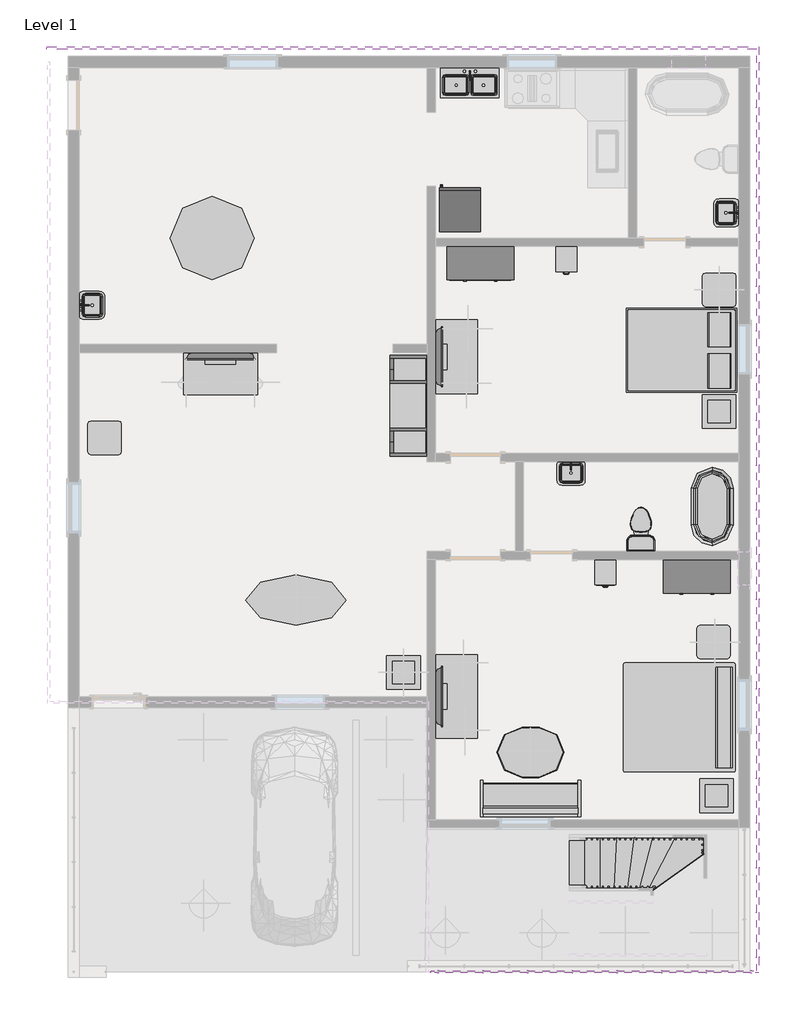
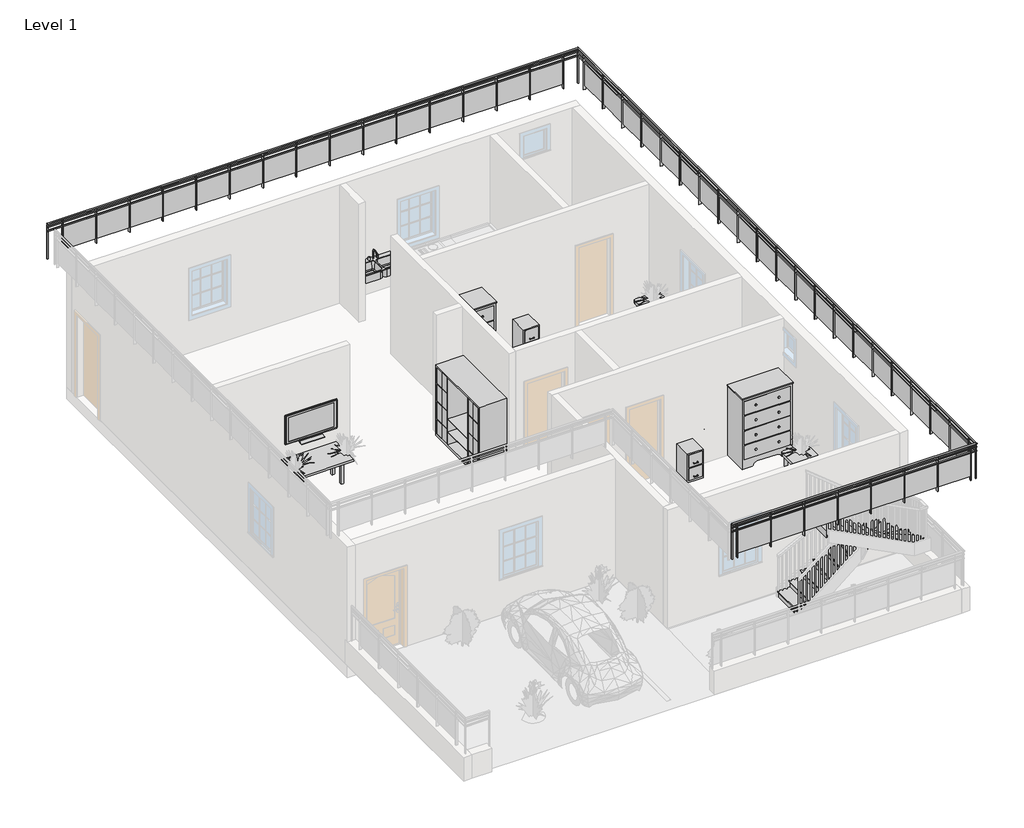
# One storey, part 4 of 5: 23 furniture elements, 7 flow terminals, 1 proxy, 1 railing, 1 stair flight.
"""IFC4 building model written with IfcOpenShell, lengths in millimetres."""

from ifc_helpers import new_model, si_unit, frame, origin, place, context, project, spatial, polyline, circle_curve, ellipse_curve, outline, extrude, faceted_brep, transform, mapped, element, save
from ifc_brep_helpers import plane_surface, cylinder_surface, advanced_brep
from components import proxy_a13a33b2, flow_terminal_accce45a, flow_terminal_a53be723, flow_terminal_62a433f7, toilet_domestic_3d_toilet_domestic_3d_f7549cf7, toilet_domestic_3d_toilet_domestic_3d_183bbd19, flow_terminal_a2f06f5b, furniture_1d2926bd, furniture_1fc5af50, furniture_bb55ed6b, furniture_9fa109b2, furniture_cf0b6580, furniture_a4ffab56, furniture_7a3aaa4f, furniture_fdf74506, furniture_b5c51a22, furniture_be1c6672, furniture_bbcc68ce, furniture_0791916c, furniture_31d08a24, furniture_48e8c7c4, furniture_2bbcfec9, stair_flight_469f198f

model = new_model("IFC4")

# Units and contexts
model_context = context("Model", 3, world=origin())
ifc_project = project(units=[si_unit("LENGTHUNIT", "METRE", prefix="MILLI")], contexts=[model_context])

# Site, building, storey
site = spatial("IfcSite", under=ifc_project)
building = spatial("IfcBuilding", under=site)
storey = spatial("IfcBuildingStorey", under=building, Name="Level 1", Elevation=0.0)

# Proxy
placement = place(None, origin())
proxy_shape = proxy_a13a33b2(model_context)
element("IfcBuildingElementProxy", 1, Name="Refrigerator : 30\" x 32\" RH", ObjectType="Refrigerator : 30\" x 32\" RH", at=placement, inside=storey, context=model_context, shape_type="MappedRepresentation", body=[
    mapped(proxy_shape, transform((-5198.8866134, 11199.3143341, 0.0), x_axis=(-1.0000000000000004, 0.0, 0.0), y_axis=(0.0, -1.0000000000000004, 0.0), z_axis=(0.0, 0.0, 1.0))),
])

# Flow terminals
flow_terminal_shape = flow_terminal_accce45a(model_context)
element("IfcFlowTerminal", 2, ObjectType="Floor Drain - Round : 5\" Strainer - 2\" Drain", at=placement, inside=storey, context=model_context, shape_type="MappedRepresentation", body=[
    mapped(flow_terminal_shape, transform((-1168.2241134, 5288.6633056, 0.0), x_axis=(1.0, 0.0, 0.0), y_axis=(0.0, 1.0, 0.0), z_axis=(0.0, 0.0, 1.0))),
])
flow_terminal_2_shape = flow_terminal_a53be723(model_context)
element("IfcFlowTerminal", 3, ObjectType="Sink Kitchen-Double : 42\" x 21\"", at=placement, inside=storey, context=model_context, shape_type="MappedRepresentation", body=[
    mapped(flow_terminal_2_shape, transform((-5032.013354, 13515.9179045, 0.0), x_axis=(1.0, 0.0, 0.0), y_axis=(0.0, 1.0, 0.0), z_axis=(0.0, 0.0, 1.0))),
])
flow_terminal_3_shape = flow_terminal_62a433f7(model_context)
element("IfcFlowTerminal", 4, ObjectType="Sink Vanity-Square : 20\" x 18\"", at=placement, inside=storey, context=model_context, shape_type="MappedRepresentation", body=[
    mapped(flow_terminal_3_shape, transform((-11935.4787123, 9463.9740651, 0.0), x_axis=(0.0, 1.0000000000000002, 0.0), y_axis=(-1.0000000000000002, 0.0, 0.0), z_axis=(0.0, 0.0, 1.0))),
])
element("IfcFlowTerminal", 5, ObjectType="Sink Vanity-Square : 20\" x 18\"", at=placement, inside=storey, context=model_context, shape_type="MappedRepresentation", body=[
    mapped(flow_terminal_3_shape, transform((-306.9695145, 11171.7525462, 0.0), x_axis=(0.0, -1.0000000000000004, 0.0), y_axis=(1.0000000000000004, 0.0, 0.0), z_axis=(0.0, 0.0, 1.0))),
])
element("IfcFlowTerminal", 6, ObjectType="Sink Vanity-Square : 20\" x 18\"", at=placement, inside=storey, context=model_context, shape_type="MappedRepresentation", body=[
    mapped(flow_terminal_3_shape, transform((-3190.513354, 6480.1179045, 0.0), x_axis=(1.0, 0.0, 0.0), y_axis=(0.0, 1.0, 0.0), z_axis=(0.0, 0.0, 1.0))),
])
toilet_domestic_3d_toilet_domestic_3d_shape = toilet_domestic_3d_toilet_domestic_3d_f7549cf7(model_context)
toilet_domestic_3d_toilet_domestic_3d_2_shape = toilet_domestic_3d_toilet_domestic_3d_183bbd19(model_context)
element("IfcFlowTerminal", 7, ObjectType="Toilet-Domestic-3D : Toilet-Domestic-3D", at=placement, inside=storey, context=model_context, shape_type="MappedRepresentation", body=[
    mapped(toilet_domestic_3d_toilet_domestic_3d_shape, transform((-1904.8241134, 5503.959333, 0.0), x_axis=(-1.0000000000000002, 0.0, 0.0), y_axis=(0.0, -1.0000000000000002, 0.0), z_axis=(0.0, 0.0, 1.0))),
    mapped(toilet_domestic_3d_toilet_domestic_3d_2_shape, transform((-1904.8241134, 5503.959333, 0.0), x_axis=(-1.0000000000000002, 0.0, 0.0), y_axis=(0.0, -1.0000000000000002, 0.0), z_axis=(0.0, 0.0, 1.0))),
])
flow_terminal_4_shape = flow_terminal_a2f06f5b(model_context)
element("IfcFlowTerminal", 8, ObjectType="Tub-Free Standing-3D : 30\" x 60\" 2", at=placement, inside=storey, context=model_context, shape_type="MappedRepresentation", body=[
    mapped(flow_terminal_4_shape, transform((-609.4241134, 5822.0633056, 0.0), x_axis=(1.0000000000000004, 0.0, 0.0), y_axis=(0.0, 1.0000000000000004, 0.0), z_axis=(0.0, 0.0, 1.0))),
])

# Furniture
furniture_shape = furniture_1d2926bd(model_context)
element("IfcFurniture", 9, ObjectType="Bed-Box : Queen 60\" x 79\"", at=placement, inside=storey, context=model_context, shape_type="MappedRepresentation", body=[
    mapped(furniture_shape, transform((-933.7946052, 8997.0633056, 0.0), x_axis=(0.0, -1.0, 0.0), y_axis=(1.0, 0.0, 0.0), z_axis=(0.0, 0.0, 1.0))),
])
furniture_2_shape = furniture_1fc5af50(model_context)
element("IfcFurniture", 10, ObjectType="Bed-Standard.0001 : King 78\" x 80\"", at=placement, inside=storey, context=model_context, shape_type="MappedRepresentation", body=[
    mapped(furniture_2_shape, transform((-1160.7290314, 2258.1518302, 0.0), x_axis=(0.0, -1.0, 0.0), y_axis=(1.0, 0.0, 0.0), z_axis=(0.0, 0.0, 1.0))),
])
furniture_3_shape = furniture_bb55ed6b(model_context)
element("IfcFurniture", 11, ObjectType="Cabinet-File 2 Drawer : 15\" x 18\"", at=placement, inside=storey, context=model_context, shape_type="MappedRepresentation", body=[
    mapped(furniture_3_shape, transform((-3135.8276664, 10459.9976058, 0.0), x_axis=(1.0, 0.0, 0.0), y_axis=(0.0, 1.0, 0.0), z_axis=(0.0, 0.0, 1.0))),
])
element("IfcFurniture", 12, ObjectType="Cabinet-File 2 Drawer : 15\" x 18\"", at=placement, inside=storey, context=model_context, shape_type="MappedRepresentation", body=[
    mapped(furniture_3_shape, transform((-2424.6276664, 4770.3976058, 0.0), x_axis=(1.0, 0.0, 0.0), y_axis=(0.0, 1.0, 0.0), z_axis=(0.0, 0.0, 1.0))),
])
furniture_4_shape = furniture_9fa109b2(model_context)
element("IfcFurniture", 13, ObjectType="Dresser : 48\" x 72\" x 24\"", at=placement, inside=storey, context=model_context, shape_type="MappedRepresentation", body=[
    mapped(furniture_4_shape, transform((-4556.6308536, 10604.8262597, 0.0), x_axis=(1.0, 0.0, 0.0), y_axis=(0.0, 1.0, 0.0), z_axis=(0.0, 0.0, 1.0))),
])
element("IfcFurniture", 14, ObjectType="Dresser : 48\" x 72\" x 24\"", at=placement, inside=storey, context=model_context, shape_type="MappedRepresentation", body=[
    mapped(furniture_4_shape, transform((-619.6308536, 4915.2262597, 0.0), x_axis=(1.0, 0.0, 0.0), y_axis=(0.0, 1.0, 0.0), z_axis=(0.0, 0.0, 1.0))),
])
furniture_5_shape = furniture_cf0b6580(model_context)
element("IfcFurniture", 15, ObjectType="Entertainment Center : 72\" x 72\" x 24\"", at=placement, inside=storey, context=model_context, shape_type="MappedRepresentation", body=[
    mapped(furniture_5_shape, transform((-5689.4241134, 7650.8633056, 0.0), x_axis=(0.0, -1.0000000000000004, 0.0), y_axis=(1.0000000000000004, 0.0, 0.0), z_axis=(0.0, 0.0, 1.0))),
])
furniture_6_shape = furniture_a4ffab56(model_context)
element("IfcFurniture", 16, ObjectType="Sofa : 72\"", at=placement, inside=storey, context=model_context, shape_type="MappedRepresentation", body=[
    mapped(furniture_6_shape, transform((-3841.0536216, 659.617404, 0.0), x_axis=(-1.0000000000000002, 0.0, 0.0), y_axis=(0.0, -1.0000000000000002, 0.0), z_axis=(0.0, 0.0, 1.0))),
])
furniture_7_shape = furniture_7a3aaa4f(model_context)
element("IfcFurniture", 17, ObjectType="TV - Flat Screen : 42\"", at=placement, inside=storey, context=model_context, shape_type="MappedRepresentation", body=[
    mapped(furniture_7_shape, transform((-5580.0854898, 8543.8078198, 990.6), x_axis=(0.0, 1.0000000000000002, 0.0), y_axis=(-1.0000000000000002, 0.0, 0.0), z_axis=(0.0, 0.0, 1.0))),
])
element("IfcFurniture", 18, ObjectType="TV - Flat Screen : 42\"", at=placement, inside=storey, context=model_context, shape_type="MappedRepresentation", body=[
    mapped(furniture_7_shape, transform((-5580.0854898, 2371.6078198, 990.6), x_axis=(0.0, 1.0000000000000002, 0.0), y_axis=(-1.0000000000000002, 0.0, 0.0), z_axis=(0.0, 0.0, 1.0))),
])
furniture_8_shape = furniture_fdf74506(model_context)
element("IfcFurniture", 19, ObjectType="TV - Flat Screen : 50\"", at=placement, inside=storey, context=model_context, shape_type="MappedRepresentation", body=[
    mapped(furniture_8_shape, transform((-9546.2795993, 8557.524682, 1041.4), x_axis=(1.0, 0.0, 0.0), y_axis=(0.0, 1.0, 0.0), z_axis=(0.0, 0.0, 1.0))),
])
furniture_9_shape = furniture_b5c51a22(model_context)
element("IfcFurniture", 20, ObjectType="Table-Coffee : 24\" x 24\" x 24\"", at=placement, inside=storey, context=model_context, shape_type="MappedRepresentation", body=[
    mapped(furniture_9_shape, transform((-500.6898801, 7454.0522278, 0.0), x_axis=(1.0, 0.0, 0.0), y_axis=(0.0, 1.0, 0.0), z_axis=(0.0, 0.0, 1.0))),
])
element("IfcFurniture", 21, ObjectType="Table-Coffee : 24\" x 24\" x 24\"", at=placement, inside=storey, context=model_context, shape_type="MappedRepresentation", body=[
    mapped(furniture_9_shape, transform((-551.4898801, 469.0522278, 0.0), x_axis=(1.0, 0.0, 0.0), y_axis=(0.0, 1.0, 0.0), z_axis=(0.0, 0.0, 1.0))),
])
element("IfcFurniture", 22, ObjectType="Table-Coffee : 24\" x 24\" x 24\"", at=placement, inside=storey, context=model_context, shape_type="MappedRepresentation", body=[
    mapped(furniture_9_shape, transform((-6241.0898801, 2710.6022278, 0.0), x_axis=(1.0, 0.0, 0.0), y_axis=(0.0, 1.0, 0.0), z_axis=(0.0, 0.0, 1.0))),
])
furniture_10_shape = furniture_be1c6672(model_context)
element("IfcFurniture", 23, ObjectType="Table-Dining Oval : 36\" x 48\"", at=placement, inside=storey, context=model_context, shape_type="MappedRepresentation", body=[
    mapped(furniture_10_shape, transform((-3509.6044413, 1709.7616663, 0.0), x_axis=(1.0, 0.0, 0.0), y_axis=(0.0, 1.0, 0.0), z_axis=(0.0, 0.0, 1.0))),
])
furniture_11_shape = furniture_bbcc68ce(model_context)
element("IfcFurniture", 24, ObjectType="Table-Dining Round w Chairs : 60\" Diameter", at=placement, inside=storey, context=model_context, shape_type="MappedRepresentation", body=[
    mapped(furniture_11_shape, transform((-9806.3060806, 10883.7419941, 0.0), x_axis=(1.0, 0.0, 0.0), y_axis=(0.0, 1.0, 0.0), z_axis=(0.0, 0.0, 1.0))),
])
furniture_12_shape = furniture_0791916c(model_context)
element("IfcFurniture", 25, ObjectType="Table-Ellipse : 72\" x 36\"", at=placement, inside=storey, context=model_context, shape_type="MappedRepresentation", body=[
    mapped(furniture_12_shape, transform((-8178.6241134, 4120.2633056, 0.0), x_axis=(1.0, 0.0, 0.0), y_axis=(0.0, 1.0, 0.0), z_axis=(0.0, 0.0, 1.0))),
])
furniture_13_shape = furniture_31d08a24(model_context)
element("IfcFurniture", 26, ObjectType="Table-End : 24\" x 24\"", at=placement, inside=storey, context=model_context, shape_type="MappedRepresentation", body=[
    mapped(furniture_13_shape, transform((-790.9577437, 9606.6633056, 0.0), x_axis=(1.0, 0.0, 0.0), y_axis=(0.0, 1.0, 0.0), z_axis=(0.0, 0.0, 1.0))),
])
element("IfcFurniture", 27, ObjectType="Table-End : 24\" x 24\"", at=placement, inside=storey, context=model_context, shape_type="MappedRepresentation", body=[
    mapped(furniture_13_shape, transform((-892.5577437, 3205.8633056, 0.0), x_axis=(1.0, 0.0, 0.0), y_axis=(0.0, 1.0, 0.0), z_axis=(0.0, 0.0, 1.0))),
])
element("IfcFurniture", 28, ObjectType="Table-End : 24\" x 24\"", at=placement, inside=storey, context=model_context, shape_type="MappedRepresentation", body=[
    mapped(furniture_13_shape, transform((-11966.9577437, 6914.2633056, 0.0), x_axis=(1.0, 0.0, 0.0), y_axis=(0.0, 1.0, 0.0), z_axis=(0.0, 0.0, 1.0))),
])
furniture_14_shape = furniture_48e8c7c4(model_context)
element("IfcFurniture", 29, ObjectType="Table-Rectangular : 72\" x 30\"", at=placement, inside=storey, context=model_context, shape_type="MappedRepresentation", body=[
    mapped(furniture_14_shape, transform((-5257.6241134, 8539.8633056, 0.0), x_axis=(0.0, 1.0000000000000002, 0.0), y_axis=(-1.0000000000000002, 0.0, 0.0), z_axis=(0.0, 0.0, 1.0))),
])
element("IfcFurniture", 30, ObjectType="Table-Rectangular : 72\" x 30\"", at=placement, inside=storey, context=model_context, shape_type="MappedRepresentation", body=[
    mapped(furniture_14_shape, transform((-9550.2241134, 8235.0633056, 0.0), x_axis=(1.0, 0.0, 0.0), y_axis=(0.0, 1.0, 0.0), z_axis=(0.0, 0.0, 1.0))),
])
furniture_15_shape = furniture_2bbcfec9(model_context)
element("IfcFurniture", 31, ObjectType="Table-Rectangular : 72\" x 30\" 2", at=placement, inside=storey, context=model_context, shape_type="MappedRepresentation", body=[
    mapped(furniture_15_shape, transform((-5257.6241134, 2367.6633056, 0.0), x_axis=(0.0, 1.0000000000000002, 0.0), y_axis=(-1.0000000000000002, 0.0, 0.0), z_axis=(0.0, 0.0, 1.0))),
])

# Railing
element("IfcRailing", 32, ObjectType="Glass Panel - Bottom Fill", at=placement, inside=storey, context=model_context, shape_type="SolidModel", body=[
    advanced_brep(
    [(-12707.5816429, 14134.2133056, 4248.15), (-12707.5816429, 14172.3133056, 4248.15), (-5722.5816429, -2617.0866944, 4248.15), (-5722.5816429, -2655.1866944, 4248.15), (201.9683571, 14134.2133056, 4248.15), (240.0683571, 14172.3133056, 4248.15), (201.9683571, -2617.0866944, 4248.15), (240.0683571, -2655.1866944, 4248.15)],
    [
        (0, 1, circle_curve(frame((-12707.5816429, 14153.2633056, 4248.15), z_axis=(-1.0, 0.0, 0.0), x_axis=(0.0, 1.0, 0.0)), 19.05)),
        (1, 0, circle_curve(frame((-12707.5816429, 14153.2633056, 4248.15), z_axis=(-1.0, 0.0, 0.0), x_axis=(0.0, 1.0, 0.0)), 19.05)),
        (2, 3, circle_curve(frame((-5722.5816429, -2636.1366944, 4248.15), z_axis=(-1.0, 0.0, 0.0), x_axis=(0.0, -1.0, 0.0)), 19.05)),
        (3, 2, circle_curve(frame((-5722.5816429, -2636.1366944, 4248.15), z_axis=(-1.0, 0.0, 0.0), x_axis=(0.0, -1.0, 0.0)), 19.05)),
        (0, 4),
        (4, 5, ellipse_curve(frame((221.0183571, 14153.2633056, 4248.15), z_axis=(-0.7071067811865459, 0.7071067811865491, 0.0), x_axis=(-0.707106781186549, -0.7071067811865458, 0.0)), 26.9407684, 19.05)),
        (5, 1),
        (5, 4, ellipse_curve(frame((221.0183571, 14153.2633056, 4248.15), z_axis=(-0.7071067811865459, 0.7071067811865491, 0.0), x_axis=(-0.707106781186549, -0.7071067811865458, 0.0)), 26.9407684, 19.05)),
        (4, 6),
        (6, 7, ellipse_curve(frame((221.0183571, -2636.1366944, 4248.15), z_axis=(0.7071067811865492, 0.7071067811865458, 0.0), x_axis=(-0.7071067811865457, 0.7071067811865495, 0.0)), 26.9407684, 19.05)),
        (7, 5),
        (7, 6, ellipse_curve(frame((221.0183571, -2636.1366944, 4248.15), z_axis=(0.7071067811865492, 0.7071067811865458, 0.0), x_axis=(-0.7071067811865457, 0.7071067811865495, 0.0)), 26.9407684, 19.05)),
        (6, 2),
        (3, 7),
    ],
    [
        plane_surface(frame((-12707.5816429, 14153.2633056, 4267.2), z_axis=(-1.0, 0.0, 0.0), x_axis=(0.0, 1.0, 0.0))),
        plane_surface(frame((-5722.5816429, -2636.1366944, 4267.2), z_axis=(-1.0, 0.0, 0.0), x_axis=(0.0, -1.0, 0.0))),
        cylinder_surface(frame((-12707.5816429, 14153.2633056, 4248.15), z_axis=(-1.0, 0.0, 0.0), x_axis=(0.0, 1.0, 0.0)), 19.05),
        cylinder_surface(frame((221.0183571, 14153.2633056, 4248.15), z_axis=(0.0, 1.0, 0.0), x_axis=(1.0, 0.0, 0.0)), 19.05),
        cylinder_surface(frame((221.0183571, -2636.1366944, 4248.15), z_axis=(1.0, 0.0, 0.0), x_axis=(0.0, -1.0, 0.0)), 19.05),
    ],
    [
        (0, [[1, 2]]),
        (1, [[3, 4]]),
        (2, [[-1, 5, 6, 7]]),
        (2, [[-2, -7, 8, -5]]),
        (3, [[-6, 9, 10, 11]]),
        (3, [[-8, -11, 12, -9]]),
        (4, [[-10, 13, -4, 14]]),
        (4, [[-12, -14, -3, -13]]),
    ],
),
    faceted_brep([(-12707.5816429, 14140.5633056, 4178.3), (-12707.5816429, 14165.9633056, 4178.3), (-12707.5816429, 14165.9633056, 4152.9), (-12707.5816429, 14140.5633056, 4152.9), (208.3183571, 14140.5633056, 4178.3), (233.7183571, 14165.9633056, 4178.3), (233.7183571, 14165.9633056, 4152.9), (208.3183571, 14140.5633056, 4152.9), (208.3183571, -2623.4366944, 4178.3), (233.7183571, -2648.8366944, 4178.3), (233.7183571, -2648.8366944, 4152.9), (208.3183571, -2623.4366944, 4152.9), (-5722.5816429, -2623.4366944, 4178.3), (-5722.5816429, -2623.4366944, 4152.9), (-5722.5816429, -2648.8366944, 4152.9), (-5722.5816429, -2648.8366944, 4178.3)], [[[0, 1, 2, 3]], [[1, 0, 4, 5]], [[2, 1, 5, 6]], [[3, 2, 6, 7]], [[0, 3, 7, 4]], [[5, 4, 8, 9]], [[6, 5, 9, 10]], [[7, 6, 10, 11]], [[4, 7, 11, 8]], [[12, 13, 14, 15]], [[9, 8, 12, 15]], [[10, 9, 15, 14]], [[11, 10, 14, 13]], [[8, 11, 13, 12]]]),
    faceted_brep([(-12707.5816429, 14140.5633056, 4076.7), (-12707.5816429, 14165.9633056, 4076.7), (-12707.5816429, 14165.9633056, 4051.3), (-12707.5816429, 14140.5633056, 4051.3), (208.3183571, 14140.5633056, 4076.7), (233.7183571, 14165.9633056, 4076.7), (233.7183571, 14165.9633056, 4051.3), (208.3183571, 14140.5633056, 4051.3), (208.3183571, -2623.4366944, 4076.7), (233.7183571, -2648.8366944, 4076.7), (233.7183571, -2648.8366944, 4051.3), (208.3183571, -2623.4366944, 4051.3), (-5722.5816429, -2623.4366944, 4076.7), (-5722.5816429, -2623.4366944, 4051.3), (-5722.5816429, -2648.8366944, 4051.3), (-5722.5816429, -2648.8366944, 4076.7)], [[[0, 1, 2, 3]], [[1, 0, 4, 5]], [[2, 1, 5, 6]], [[3, 2, 6, 7]], [[0, 3, 7, 4]], [[5, 4, 8, 9]], [[6, 5, 9, 10]], [[7, 6, 10, 11]], [[4, 7, 11, 8]], [[12, 13, 14, 15]], [[9, 8, 12, 15]], [[10, 9, 15, 14]], [[11, 10, 14, 13]], [[8, 11, 13, 12]]]),
    extrude(outline(polyline([(-5589.2316429, -2610.7366944), (-5589.2316429, -2661.5366944), (-5601.9316429, -2661.5366944), (-5601.9316429, -2610.7366944), (-5589.2316429, -2610.7366944)])), frame((0.0, 0.0, 3352.8), z_axis=(0.0, 0.0, 1.0), x_axis=(1.0, 0.0, 0.0)), (0.0, 0.0, 1.0), 876.3),
    extrude(outline(polyline([(-4782.7816429, -2642.6718514), (-5595.5816429, -2642.6718514), (-5595.5816429, -2636.3218514), (-4782.7816429, -2636.3218514), (-4782.7816429, -2642.6718514)])), frame((0.0, 0.0, 3454.4), z_axis=(0.0, 0.0, 1.0), x_axis=(1.0, 0.0, 0.0)), (0.0, 0.0, 1.0), 596.9),
    extrude(outline(polyline([(-4776.4316429, -2610.7366944), (-4776.4316429, -2661.5366944), (-4789.1316429, -2661.5366944), (-4789.1316429, -2610.7366944), (-4776.4316429, -2610.7366944)])), frame((0.0, 0.0, 3352.8), z_axis=(0.0, 0.0, 1.0), x_axis=(1.0, 0.0, 0.0)), (0.0, 0.0, 1.0), 876.3),
    extrude(outline(polyline([(-3969.9816429, -2642.6718514), (-4782.7816429, -2642.6718514), (-4782.7816429, -2636.3218514), (-3969.9816429, -2636.3218514), (-3969.9816429, -2642.6718514)])), frame((0.0, 0.0, 3454.4), z_axis=(0.0, 0.0, 1.0), x_axis=(1.0, 0.0, 0.0)), (0.0, 0.0, 1.0), 596.9),
    extrude(outline(polyline([(-3963.6316429, -2610.7366944), (-3963.6316429, -2661.5366944), (-3976.3316429, -2661.5366944), (-3976.3316429, -2610.7366944), (-3963.6316429, -2610.7366944)])), frame((0.0, 0.0, 3352.8), z_axis=(0.0, 0.0, 1.0), x_axis=(1.0, 0.0, 0.0)), (0.0, 0.0, 1.0), 876.3),
    extrude(outline(polyline([(-3157.1816429, -2642.6718514), (-3969.9816429, -2642.6718514), (-3969.9816429, -2636.3218514), (-3157.1816429, -2636.3218514), (-3157.1816429, -2642.6718514)])), frame((0.0, 0.0, 3454.4), z_axis=(0.0, 0.0, 1.0), x_axis=(1.0, 0.0, 0.0)), (0.0, 0.0, 1.0), 596.9),
    extrude(outline(polyline([(-3150.8316429, -2610.7366944), (-3150.8316429, -2661.5366944), (-3163.5316429, -2661.5366944), (-3163.5316429, -2610.7366944), (-3150.8316429, -2610.7366944)])), frame((0.0, 0.0, 3352.8), z_axis=(0.0, 0.0, 1.0), x_axis=(1.0, 0.0, 0.0)), (0.0, 0.0, 1.0), 876.3),
    extrude(outline(polyline([(-2344.3816429, -2642.6718514), (-3157.1816429, -2642.6718514), (-3157.1816429, -2636.3218514), (-2344.3816429, -2636.3218514), (-2344.3816429, -2642.6718514)])), frame((0.0, 0.0, 3454.4), z_axis=(0.0, 0.0, 1.0), x_axis=(1.0, 0.0, 0.0)), (0.0, 0.0, 1.0), 596.9),
    extrude(outline(polyline([(-2338.0316429, -2610.7366944), (-2338.0316429, -2661.5366944), (-2350.7316429, -2661.5366944), (-2350.7316429, -2610.7366944), (-2338.0316429, -2610.7366944)])), frame((0.0, 0.0, 3352.8), z_axis=(0.0, 0.0, 1.0), x_axis=(1.0, 0.0, 0.0)), (0.0, 0.0, 1.0), 876.3),
    extrude(outline(polyline([(-1531.5816429, -2642.6718514), (-2344.3816429, -2642.6718514), (-2344.3816429, -2636.3218514), (-1531.5816429, -2636.3218514), (-1531.5816429, -2642.6718514)])), frame((0.0, 0.0, 3454.4), z_axis=(0.0, 0.0, 1.0), x_axis=(1.0, 0.0, 0.0)), (0.0, 0.0, 1.0), 596.9),
    extrude(outline(polyline([(-1525.2316429, -2610.7366944), (-1525.2316429, -2661.5366944), (-1537.9316429, -2661.5366944), (-1537.9316429, -2610.7366944), (-1525.2316429, -2610.7366944)])), frame((0.0, 0.0, 3352.8), z_axis=(0.0, 0.0, 1.0), x_axis=(1.0, 0.0, 0.0)), (0.0, 0.0, 1.0), 876.3),
    extrude(outline(polyline([(-718.7816429, -2642.6718514), (-1531.5816429, -2642.6718514), (-1531.5816429, -2636.3218514), (-718.7816429, -2636.3218514), (-718.7816429, -2642.6718514)])), frame((0.0, 0.0, 3454.4), z_axis=(0.0, 0.0, 1.0), x_axis=(1.0, 0.0, 0.0)), (0.0, 0.0, 1.0), 596.9),
    extrude(outline(polyline([(-712.4316429, -2610.7366944), (-712.4316429, -2661.5366944), (-725.1316429, -2661.5366944), (-725.1316429, -2610.7366944), (-712.4316429, -2610.7366944)])), frame((0.0, 0.0, 3352.8), z_axis=(0.0, 0.0, 1.0), x_axis=(1.0, 0.0, 0.0)), (0.0, 0.0, 1.0), 876.3),
    extrude(outline(polyline([(94.0183571, -2642.6718514), (-718.7816429, -2642.6718514), (-718.7816429, -2636.3218514), (94.0183571, -2636.3218514), (94.0183571, -2642.6718514)])), frame((0.0, 0.0, 3454.4), z_axis=(0.0, 0.0, 1.0), x_axis=(1.0, 0.0, 0.0)), (0.0, 0.0, 1.0), 596.9),
    extrude(outline(polyline([(100.3683571, -2610.7366944), (100.3683571, -2661.5366944), (87.6683571, -2661.5366944), (87.6683571, -2610.7366944), (100.3683571, -2610.7366944)])), frame((0.0, 0.0, 3352.8), z_axis=(0.0, 0.0, 1.0), x_axis=(1.0, 0.0, 0.0)), (0.0, 0.0, 1.0), 876.3),
    extrude(outline(polyline([(195.6183571, -2363.0866944), (246.4183571, -2363.0866944), (246.4183571, -2375.7866944), (195.6183571, -2375.7866944), (195.6183571, -2363.0866944)])), frame((0.0, 0.0, 3352.8), z_axis=(0.0, 0.0, 1.0), x_axis=(1.0, 0.0, 0.0)), (0.0, 0.0, 1.0), 876.3),
    extrude(outline(polyline([(227.5535141, -1556.6366944), (227.5535141, -2369.4366944), (221.2035141, -2369.4366944), (221.2035141, -1556.6366944), (227.5535141, -1556.6366944)])), frame((0.0, 0.0, 3454.4), z_axis=(0.0, 0.0, 1.0), x_axis=(1.0, 0.0, 0.0)), (0.0, 0.0, 1.0), 596.9),
    extrude(outline(polyline([(195.6183571, -1550.2866944), (246.4183571, -1550.2866944), (246.4183571, -1562.9866944), (195.6183571, -1562.9866944), (195.6183571, -1550.2866944)])), frame((0.0, 0.0, 3352.8), z_axis=(0.0, 0.0, 1.0), x_axis=(1.0, 0.0, 0.0)), (0.0, 0.0, 1.0), 876.3),
    extrude(outline(polyline([(227.5535141, -743.8366944), (227.5535141, -1556.6366944), (221.2035141, -1556.6366944), (221.2035141, -743.8366944), (227.5535141, -743.8366944)])), frame((0.0, 0.0, 3454.4), z_axis=(0.0, 0.0, 1.0), x_axis=(1.0, 0.0, 0.0)), (0.0, 0.0, 1.0), 596.9),
    extrude(outline(polyline([(195.6183571, -737.4866944), (246.4183571, -737.4866944), (246.4183571, -750.1866944), (195.6183571, -750.1866944), (195.6183571, -737.4866944)])), frame((0.0, 0.0, 3352.8), z_axis=(0.0, 0.0, 1.0), x_axis=(1.0, 0.0, 0.0)), (0.0, 0.0, 1.0), 876.3),
    extrude(outline(polyline([(227.5535141, 68.9633056), (227.5535141, -743.8366944), (221.2035141, -743.8366944), (221.2035141, 68.9633056), (227.5535141, 68.9633056)])), frame((0.0, 0.0, 3454.4), z_axis=(0.0, 0.0, 1.0), x_axis=(1.0, 0.0, 0.0)), (0.0, 0.0, 1.0), 596.9),
    extrude(outline(polyline([(195.6183571, 75.3133056), (246.4183571, 75.3133056), (246.4183571, 62.6133056), (195.6183571, 62.6133056), (195.6183571, 75.3133056)])), frame((0.0, 0.0, 3352.8), z_axis=(0.0, 0.0, 1.0), x_axis=(1.0, 0.0, 0.0)), (0.0, 0.0, 1.0), 876.3),
    extrude(outline(polyline([(227.5535141, 881.7633056), (227.5535141, 68.9633056), (221.2035141, 68.9633056), (221.2035141, 881.7633056), (227.5535141, 881.7633056)])), frame((0.0, 0.0, 3454.4), z_axis=(0.0, 0.0, 1.0), x_axis=(1.0, 0.0, 0.0)), (0.0, 0.0, 1.0), 596.9),
    extrude(outline(polyline([(195.6183571, 888.1133056), (246.4183571, 888.1133056), (246.4183571, 875.4133056), (195.6183571, 875.4133056), (195.6183571, 888.1133056)])), frame((0.0, 0.0, 3352.8), z_axis=(0.0, 0.0, 1.0), x_axis=(1.0, 0.0, 0.0)), (0.0, 0.0, 1.0), 876.3),
    extrude(outline(polyline([(227.5535141, 1694.5633056), (227.5535141, 881.7633056), (221.2035141, 881.7633056), (221.2035141, 1694.5633056), (227.5535141, 1694.5633056)])), frame((0.0, 0.0, 3454.4), z_axis=(0.0, 0.0, 1.0), x_axis=(1.0, 0.0, 0.0)), (0.0, 0.0, 1.0), 596.9),
    extrude(outline(polyline([(195.6183571, 1700.9133056), (246.4183571, 1700.9133056), (246.4183571, 1688.2133056), (195.6183571, 1688.2133056), (195.6183571, 1700.9133056)])), frame((0.0, 0.0, 3352.8), z_axis=(0.0, 0.0, 1.0), x_axis=(1.0, 0.0, 0.0)), (0.0, 0.0, 1.0), 876.3),
    extrude(outline(polyline([(227.5535141, 2507.3633056), (227.5535141, 1694.5633056), (221.2035141, 1694.5633056), (221.2035141, 2507.3633056), (227.5535141, 2507.3633056)])), frame((0.0, 0.0, 3454.4), z_axis=(0.0, 0.0, 1.0), x_axis=(1.0, 0.0, 0.0)), (0.0, 0.0, 1.0), 596.9),
    extrude(outline(polyline([(195.6183571, 2513.7133056), (246.4183571, 2513.7133056), (246.4183571, 2501.0133056), (195.6183571, 2501.0133056), (195.6183571, 2513.7133056)])), frame((0.0, 0.0, 3352.8), z_axis=(0.0, 0.0, 1.0), x_axis=(1.0, 0.0, 0.0)), (0.0, 0.0, 1.0), 876.3),
    extrude(outline(polyline([(227.5535141, 3320.1633056), (227.5535141, 2507.3633056), (221.2035141, 2507.3633056), (221.2035141, 3320.1633056), (227.5535141, 3320.1633056)])), frame((0.0, 0.0, 3454.4), z_axis=(0.0, 0.0, 1.0), x_axis=(1.0, 0.0, 0.0)), (0.0, 0.0, 1.0), 596.9),
    extrude(outline(polyline([(195.6183571, 3326.5133056), (246.4183571, 3326.5133056), (246.4183571, 3313.8133056), (195.6183571, 3313.8133056), (195.6183571, 3326.5133056)])), frame((0.0, 0.0, 3352.8), z_axis=(0.0, 0.0, 1.0), x_axis=(1.0, 0.0, 0.0)), (0.0, 0.0, 1.0), 876.3),
    extrude(outline(polyline([(227.5535141, 4132.9633056), (227.5535141, 3320.1633056), (221.2035141, 3320.1633056), (221.2035141, 4132.9633056), (227.5535141, 4132.9633056)])), frame((0.0, 0.0, 3454.4), z_axis=(0.0, 0.0, 1.0), x_axis=(1.0, 0.0, 0.0)), (0.0, 0.0, 1.0), 596.9),
    extrude(outline(polyline([(195.6183571, 4139.3133056), (246.4183571, 4139.3133056), (246.4183571, 4126.6133056), (195.6183571, 4126.6133056), (195.6183571, 4139.3133056)])), frame((0.0, 0.0, 3352.8), z_axis=(0.0, 0.0, 1.0), x_axis=(1.0, 0.0, 0.0)), (0.0, 0.0, 1.0), 876.3),
    extrude(outline(polyline([(227.5535141, 4945.7633056), (227.5535141, 4132.9633056), (221.2035141, 4132.9633056), (221.2035141, 4945.7633056), (227.5535141, 4945.7633056)])), frame((0.0, 0.0, 3454.4), z_axis=(0.0, 0.0, 1.0), x_axis=(1.0, 0.0, 0.0)), (0.0, 0.0, 1.0), 596.9),
    extrude(outline(polyline([(195.6183571, 4952.1133056), (246.4183571, 4952.1133056), (246.4183571, 4939.4133056), (195.6183571, 4939.4133056), (195.6183571, 4952.1133056)])), frame((0.0, 0.0, 3352.8), z_axis=(0.0, 0.0, 1.0), x_axis=(1.0, 0.0, 0.0)), (0.0, 0.0, 1.0), 876.3),
    extrude(outline(polyline([(227.5535141, 5758.5633056), (227.5535141, 4945.7633056), (221.2035141, 4945.7633056), (221.2035141, 5758.5633056), (227.5535141, 5758.5633056)])), frame((0.0, 0.0, 3454.4), z_axis=(0.0, 0.0, 1.0), x_axis=(1.0, 0.0, 0.0)), (0.0, 0.0, 1.0), 596.9),
    extrude(outline(polyline([(195.6183571, 5764.9133056), (246.4183571, 5764.9133056), (246.4183571, 5752.2133056), (195.6183571, 5752.2133056), (195.6183571, 5764.9133056)])), frame((0.0, 0.0, 3352.8), z_axis=(0.0, 0.0, 1.0), x_axis=(1.0, 0.0, 0.0)), (0.0, 0.0, 1.0), 876.3),
    extrude(outline(polyline([(227.5535141, 6571.3633056), (227.5535141, 5758.5633056), (221.2035141, 5758.5633056), (221.2035141, 6571.3633056), (227.5535141, 6571.3633056)])), frame((0.0, 0.0, 3454.4), z_axis=(0.0, 0.0, 1.0), x_axis=(1.0, 0.0, 0.0)), (0.0, 0.0, 1.0), 596.9),
    extrude(outline(polyline([(195.6183571, 6577.7133056), (246.4183571, 6577.7133056), (246.4183571, 6565.0133056), (195.6183571, 6565.0133056), (195.6183571, 6577.7133056)])), frame((0.0, 0.0, 3352.8), z_axis=(0.0, 0.0, 1.0), x_axis=(1.0, 0.0, 0.0)), (0.0, 0.0, 1.0), 876.3),
    extrude(outline(polyline([(227.5535141, 7384.1633056), (227.5535141, 6571.3633056), (221.2035141, 6571.3633056), (221.2035141, 7384.1633056), (227.5535141, 7384.1633056)])), frame((0.0, 0.0, 3454.4), z_axis=(0.0, 0.0, 1.0), x_axis=(1.0, 0.0, 0.0)), (0.0, 0.0, 1.0), 596.9),
    extrude(outline(polyline([(195.6183571, 7390.5133056), (246.4183571, 7390.5133056), (246.4183571, 7377.8133056), (195.6183571, 7377.8133056), (195.6183571, 7390.5133056)])), frame((0.0, 0.0, 3352.8), z_axis=(0.0, 0.0, 1.0), x_axis=(1.0, 0.0, 0.0)), (0.0, 0.0, 1.0), 876.3),
    extrude(outline(polyline([(227.5535141, 8196.9633056), (227.5535141, 7384.1633056), (221.2035141, 7384.1633056), (221.2035141, 8196.9633056), (227.5535141, 8196.9633056)])), frame((0.0, 0.0, 3454.4), z_axis=(0.0, 0.0, 1.0), x_axis=(1.0, 0.0, 0.0)), (0.0, 0.0, 1.0), 596.9),
    extrude(outline(polyline([(195.6183571, 8203.3133056), (246.4183571, 8203.3133056), (246.4183571, 8190.6133056), (195.6183571, 8190.6133056), (195.6183571, 8203.3133056)])), frame((0.0, 0.0, 3352.8), z_axis=(0.0, 0.0, 1.0), x_axis=(1.0, 0.0, 0.0)), (0.0, 0.0, 1.0), 876.3),
    extrude(outline(polyline([(227.5535141, 9009.7633056), (227.5535141, 8196.9633056), (221.2035141, 8196.9633056), (221.2035141, 9009.7633056), (227.5535141, 9009.7633056)])), frame((0.0, 0.0, 3454.4), z_axis=(0.0, 0.0, 1.0), x_axis=(1.0, 0.0, 0.0)), (0.0, 0.0, 1.0), 596.9),
    extrude(outline(polyline([(195.6183571, 9016.1133056), (246.4183571, 9016.1133056), (246.4183571, 9003.4133056), (195.6183571, 9003.4133056), (195.6183571, 9016.1133056)])), frame((0.0, 0.0, 3352.8), z_axis=(0.0, 0.0, 1.0), x_axis=(1.0, 0.0, 0.0)), (0.0, 0.0, 1.0), 876.3),
    extrude(outline(polyline([(227.5535141, 9822.5633056), (227.5535141, 9009.7633056), (221.2035141, 9009.7633056), (221.2035141, 9822.5633056), (227.5535141, 9822.5633056)])), frame((0.0, 0.0, 3454.4), z_axis=(0.0, 0.0, 1.0), x_axis=(1.0, 0.0, 0.0)), (0.0, 0.0, 1.0), 596.9),
    extrude(outline(polyline([(195.6183571, 9828.9133056), (246.4183571, 9828.9133056), (246.4183571, 9816.2133056), (195.6183571, 9816.2133056), (195.6183571, 9828.9133056)])), frame((0.0, 0.0, 3352.8), z_axis=(0.0, 0.0, 1.0), x_axis=(1.0, 0.0, 0.0)), (0.0, 0.0, 1.0), 876.3),
    extrude(outline(polyline([(227.5535141, 10635.3633056), (227.5535141, 9822.5633056), (221.2035141, 9822.5633056), (221.2035141, 10635.3633056), (227.5535141, 10635.3633056)])), frame((0.0, 0.0, 3454.4), z_axis=(0.0, 0.0, 1.0), x_axis=(1.0, 0.0, 0.0)), (0.0, 0.0, 1.0), 596.9),
    extrude(outline(polyline([(195.6183571, 10641.7133056), (246.4183571, 10641.7133056), (246.4183571, 10629.0133056), (195.6183571, 10629.0133056), (195.6183571, 10641.7133056)])), frame((0.0, 0.0, 3352.8), z_axis=(0.0, 0.0, 1.0), x_axis=(1.0, 0.0, 0.0)), (0.0, 0.0, 1.0), 876.3),
    extrude(outline(polyline([(227.5535141, 11448.1633056), (227.5535141, 10635.3633056), (221.2035141, 10635.3633056), (221.2035141, 11448.1633056), (227.5535141, 11448.1633056)])), frame((0.0, 0.0, 3454.4), z_axis=(0.0, 0.0, 1.0), x_axis=(1.0, 0.0, 0.0)), (0.0, 0.0, 1.0), 596.9),
    extrude(outline(polyline([(195.6183571, 11454.5133056), (246.4183571, 11454.5133056), (246.4183571, 11441.8133056), (195.6183571, 11441.8133056), (195.6183571, 11454.5133056)])), frame((0.0, 0.0, 3352.8), z_axis=(0.0, 0.0, 1.0), x_axis=(1.0, 0.0, 0.0)), (0.0, 0.0, 1.0), 876.3),
    extrude(outline(polyline([(227.5535141, 12260.9633056), (227.5535141, 11448.1633056), (221.2035141, 11448.1633056), (221.2035141, 12260.9633056), (227.5535141, 12260.9633056)])), frame((0.0, 0.0, 3454.4), z_axis=(0.0, 0.0, 1.0), x_axis=(1.0, 0.0, 0.0)), (0.0, 0.0, 1.0), 596.9),
    extrude(outline(polyline([(195.6183571, 12267.3133056), (246.4183571, 12267.3133056), (246.4183571, 12254.6133056), (195.6183571, 12254.6133056), (195.6183571, 12267.3133056)])), frame((0.0, 0.0, 3352.8), z_axis=(0.0, 0.0, 1.0), x_axis=(1.0, 0.0, 0.0)), (0.0, 0.0, 1.0), 876.3),
    extrude(outline(polyline([(227.5535141, 13073.7633056), (227.5535141, 12260.9633056), (221.2035141, 12260.9633056), (221.2035141, 13073.7633056), (227.5535141, 13073.7633056)])), frame((0.0, 0.0, 3454.4), z_axis=(0.0, 0.0, 1.0), x_axis=(1.0, 0.0, 0.0)), (0.0, 0.0, 1.0), 596.9),
    extrude(outline(polyline([(195.6183571, 13080.1133056), (246.4183571, 13080.1133056), (246.4183571, 13067.4133056), (195.6183571, 13067.4133056), (195.6183571, 13080.1133056)])), frame((0.0, 0.0, 3352.8), z_axis=(0.0, 0.0, 1.0), x_axis=(1.0, 0.0, 0.0)), (0.0, 0.0, 1.0), 876.3),
    extrude(outline(polyline([(227.5535141, 13886.5633056), (227.5535141, 13073.7633056), (221.2035141, 13073.7633056), (221.2035141, 13886.5633056), (227.5535141, 13886.5633056)])), frame((0.0, 0.0, 3454.4), z_axis=(0.0, 0.0, 1.0), x_axis=(1.0, 0.0, 0.0)), (0.0, 0.0, 1.0), 596.9),
    extrude(outline(polyline([(195.6183571, 13892.9133056), (246.4183571, 13892.9133056), (246.4183571, 13880.2133056), (195.6183571, 13880.2133056), (195.6183571, 13892.9133056)])), frame((0.0, 0.0, 3352.8), z_axis=(0.0, 0.0, 1.0), x_axis=(1.0, 0.0, 0.0)), (0.0, 0.0, 1.0), 876.3),
    extrude(outline(polyline([(-153.6316429, 14127.8633056), (-153.6316429, 14178.6633056), (-140.9316429, 14178.6633056), (-140.9316429, 14127.8633056), (-153.6316429, 14127.8633056)])), frame((0.0, 0.0, 3352.8), z_axis=(0.0, 0.0, 1.0), x_axis=(1.0, 0.0, 0.0)), (0.0, 0.0, 1.0), 876.3),
    extrude(outline(polyline([(-960.0816429, 14159.7984626), (-147.2816429, 14159.7984626), (-147.2816429, 14153.4484626), (-960.0816429, 14153.4484626), (-960.0816429, 14159.7984626)])), frame((0.0, 0.0, 3454.4), z_axis=(0.0, 0.0, 1.0), x_axis=(1.0, 0.0, 0.0)), (0.0, 0.0, 1.0), 596.9),
    extrude(outline(polyline([(-966.4316429, 14127.8633056), (-966.4316429, 14178.6633056), (-953.7316429, 14178.6633056), (-953.7316429, 14127.8633056), (-966.4316429, 14127.8633056)])), frame((0.0, 0.0, 3352.8), z_axis=(0.0, 0.0, 1.0), x_axis=(1.0, 0.0, 0.0)), (0.0, 0.0, 1.0), 876.3),
    extrude(outline(polyline([(-1772.8816429, 14159.7984626), (-960.0816429, 14159.7984626), (-960.0816429, 14153.4484626), (-1772.8816429, 14153.4484626), (-1772.8816429, 14159.7984626)])), frame((0.0, 0.0, 3454.4), z_axis=(0.0, 0.0, 1.0), x_axis=(1.0, 0.0, 0.0)), (0.0, 0.0, 1.0), 596.9),
    extrude(outline(polyline([(-1779.2316429, 14127.8633056), (-1779.2316429, 14178.6633056), (-1766.5316429, 14178.6633056), (-1766.5316429, 14127.8633056), (-1779.2316429, 14127.8633056)])), frame((0.0, 0.0, 3352.8), z_axis=(0.0, 0.0, 1.0), x_axis=(1.0, 0.0, 0.0)), (0.0, 0.0, 1.0), 876.3),
    extrude(outline(polyline([(-2585.6816429, 14159.7984626), (-1772.8816429, 14159.7984626), (-1772.8816429, 14153.4484626), (-2585.6816429, 14153.4484626), (-2585.6816429, 14159.7984626)])), frame((0.0, 0.0, 3454.4), z_axis=(0.0, 0.0, 1.0), x_axis=(1.0, 0.0, 0.0)), (0.0, 0.0, 1.0), 596.9),
    extrude(outline(polyline([(-2592.0316429, 14127.8633056), (-2592.0316429, 14178.6633056), (-2579.3316429, 14178.6633056), (-2579.3316429, 14127.8633056), (-2592.0316429, 14127.8633056)])), frame((0.0, 0.0, 3352.8), z_axis=(0.0, 0.0, 1.0), x_axis=(1.0, 0.0, 0.0)), (0.0, 0.0, 1.0), 876.3),
    extrude(outline(polyline([(-3398.4816429, 14159.7984626), (-2585.6816429, 14159.7984626), (-2585.6816429, 14153.4484626), (-3398.4816429, 14153.4484626), (-3398.4816429, 14159.7984626)])), frame((0.0, 0.0, 3454.4), z_axis=(0.0, 0.0, 1.0), x_axis=(1.0, 0.0, 0.0)), (0.0, 0.0, 1.0), 596.9),
    extrude(outline(polyline([(-3404.8316429, 14127.8633056), (-3404.8316429, 14178.6633056), (-3392.1316429, 14178.6633056), (-3392.1316429, 14127.8633056), (-3404.8316429, 14127.8633056)])), frame((0.0, 0.0, 3352.8), z_axis=(0.0, 0.0, 1.0), x_axis=(1.0, 0.0, 0.0)), (0.0, 0.0, 1.0), 876.3),
    extrude(outline(polyline([(-4211.2816429, 14159.7984626), (-3398.4816429, 14159.7984626), (-3398.4816429, 14153.4484626), (-4211.2816429, 14153.4484626), (-4211.2816429, 14159.7984626)])), frame((0.0, 0.0, 3454.4), z_axis=(0.0, 0.0, 1.0), x_axis=(1.0, 0.0, 0.0)), (0.0, 0.0, 1.0), 596.9),
    extrude(outline(polyline([(-4217.6316429, 14127.8633056), (-4217.6316429, 14178.6633056), (-4204.9316429, 14178.6633056), (-4204.9316429, 14127.8633056), (-4217.6316429, 14127.8633056)])), frame((0.0, 0.0, 3352.8), z_axis=(0.0, 0.0, 1.0), x_axis=(1.0, 0.0, 0.0)), (0.0, 0.0, 1.0), 876.3),
    extrude(outline(polyline([(-5024.0816429, 14159.7984626), (-4211.2816429, 14159.7984626), (-4211.2816429, 14153.4484626), (-5024.0816429, 14153.4484626), (-5024.0816429, 14159.7984626)])), frame((0.0, 0.0, 3454.4), z_axis=(0.0, 0.0, 1.0), x_axis=(1.0, 0.0, 0.0)), (0.0, 0.0, 1.0), 596.9),
    extrude(outline(polyline([(-5030.4316429, 14127.8633056), (-5030.4316429, 14178.6633056), (-5017.7316429, 14178.6633056), (-5017.7316429, 14127.8633056), (-5030.4316429, 14127.8633056)])), frame((0.0, 0.0, 3352.8), z_axis=(0.0, 0.0, 1.0), x_axis=(1.0, 0.0, 0.0)), (0.0, 0.0, 1.0), 876.3),
    extrude(outline(polyline([(-5836.8816429, 14159.7984626), (-5024.0816429, 14159.7984626), (-5024.0816429, 14153.4484626), (-5836.8816429, 14153.4484626), (-5836.8816429, 14159.7984626)])), frame((0.0, 0.0, 3454.4), z_axis=(0.0, 0.0, 1.0), x_axis=(1.0, 0.0, 0.0)), (0.0, 0.0, 1.0), 596.9),
    extrude(outline(polyline([(-5843.2316429, 14127.8633056), (-5843.2316429, 14178.6633056), (-5830.5316429, 14178.6633056), (-5830.5316429, 14127.8633056), (-5843.2316429, 14127.8633056)])), frame((0.0, 0.0, 3352.8), z_axis=(0.0, 0.0, 1.0), x_axis=(1.0, 0.0, 0.0)), (0.0, 0.0, 1.0), 876.3),
    extrude(outline(polyline([(-6649.6816429, 14159.7984626), (-5836.8816429, 14159.7984626), (-5836.8816429, 14153.4484626), (-6649.6816429, 14153.4484626), (-6649.6816429, 14159.7984626)])), frame((0.0, 0.0, 3454.4), z_axis=(0.0, 0.0, 1.0), x_axis=(1.0, 0.0, 0.0)), (0.0, 0.0, 1.0), 596.9),
    extrude(outline(polyline([(-6656.0316429, 14127.8633056), (-6656.0316429, 14178.6633056), (-6643.3316429, 14178.6633056), (-6643.3316429, 14127.8633056), (-6656.0316429, 14127.8633056)])), frame((0.0, 0.0, 3352.8), z_axis=(0.0, 0.0, 1.0), x_axis=(1.0, 0.0, 0.0)), (0.0, 0.0, 1.0), 876.3),
    extrude(outline(polyline([(-7462.4816429, 14159.7984626), (-6649.6816429, 14159.7984626), (-6649.6816429, 14153.4484626), (-7462.4816429, 14153.4484626), (-7462.4816429, 14159.7984626)])), frame((0.0, 0.0, 3454.4), z_axis=(0.0, 0.0, 1.0), x_axis=(1.0, 0.0, 0.0)), (0.0, 0.0, 1.0), 596.9),
    extrude(outline(polyline([(-7468.8316429, 14127.8633056), (-7468.8316429, 14178.6633056), (-7456.1316429, 14178.6633056), (-7456.1316429, 14127.8633056), (-7468.8316429, 14127.8633056)])), frame((0.0, 0.0, 3352.8), z_axis=(0.0, 0.0, 1.0), x_axis=(1.0, 0.0, 0.0)), (0.0, 0.0, 1.0), 876.3),
    extrude(outline(polyline([(-8275.2816429, 14159.7984626), (-7462.4816429, 14159.7984626), (-7462.4816429, 14153.4484626), (-8275.2816429, 14153.4484626), (-8275.2816429, 14159.7984626)])), frame((0.0, 0.0, 3454.4), z_axis=(0.0, 0.0, 1.0), x_axis=(1.0, 0.0, 0.0)), (0.0, 0.0, 1.0), 596.9),
    extrude(outline(polyline([(-8281.6316429, 14127.8633056), (-8281.6316429, 14178.6633056), (-8268.9316429, 14178.6633056), (-8268.9316429, 14127.8633056), (-8281.6316429, 14127.8633056)])), frame((0.0, 0.0, 3352.8), z_axis=(0.0, 0.0, 1.0), x_axis=(1.0, 0.0, 0.0)), (0.0, 0.0, 1.0), 876.3),
    extrude(outline(polyline([(-9088.0816429, 14159.7984626), (-8275.2816429, 14159.7984626), (-8275.2816429, 14153.4484626), (-9088.0816429, 14153.4484626), (-9088.0816429, 14159.7984626)])), frame((0.0, 0.0, 3454.4), z_axis=(0.0, 0.0, 1.0), x_axis=(1.0, 0.0, 0.0)), (0.0, 0.0, 1.0), 596.9),
    extrude(outline(polyline([(-9094.4316429, 14127.8633056), (-9094.4316429, 14178.6633056), (-9081.7316429, 14178.6633056), (-9081.7316429, 14127.8633056), (-9094.4316429, 14127.8633056)])), frame((0.0, 0.0, 3352.8), z_axis=(0.0, 0.0, 1.0), x_axis=(1.0, 0.0, 0.0)), (0.0, 0.0, 1.0), 876.3),
    extrude(outline(polyline([(-9900.8816429, 14159.7984626), (-9088.0816429, 14159.7984626), (-9088.0816429, 14153.4484626), (-9900.8816429, 14153.4484626), (-9900.8816429, 14159.7984626)])), frame((0.0, 0.0, 3454.4), z_axis=(0.0, 0.0, 1.0), x_axis=(1.0, 0.0, 0.0)), (0.0, 0.0, 1.0), 596.9),
    extrude(outline(polyline([(-9907.2316429, 14127.8633056), (-9907.2316429, 14178.6633056), (-9894.5316429, 14178.6633056), (-9894.5316429, 14127.8633056), (-9907.2316429, 14127.8633056)])), frame((0.0, 0.0, 3352.8), z_axis=(0.0, 0.0, 1.0), x_axis=(1.0, 0.0, 0.0)), (0.0, 0.0, 1.0), 876.3),
    extrude(outline(polyline([(-10713.6816429, 14159.7984626), (-9900.8816429, 14159.7984626), (-9900.8816429, 14153.4484626), (-10713.6816429, 14153.4484626), (-10713.6816429, 14159.7984626)])), frame((0.0, 0.0, 3454.4), z_axis=(0.0, 0.0, 1.0), x_axis=(1.0, 0.0, 0.0)), (0.0, 0.0, 1.0), 596.9),
    extrude(outline(polyline([(-10720.0316429, 14127.8633056), (-10720.0316429, 14178.6633056), (-10707.3316429, 14178.6633056), (-10707.3316429, 14127.8633056), (-10720.0316429, 14127.8633056)])), frame((0.0, 0.0, 3352.8), z_axis=(0.0, 0.0, 1.0), x_axis=(1.0, 0.0, 0.0)), (0.0, 0.0, 1.0), 876.3),
    extrude(outline(polyline([(-11526.4816429, 14159.7984626), (-10713.6816429, 14159.7984626), (-10713.6816429, 14153.4484626), (-11526.4816429, 14153.4484626), (-11526.4816429, 14159.7984626)])), frame((0.0, 0.0, 3454.4), z_axis=(0.0, 0.0, 1.0), x_axis=(1.0, 0.0, 0.0)), (0.0, 0.0, 1.0), 596.9),
    extrude(outline(polyline([(-11532.8316429, 14127.8633056), (-11532.8316429, 14178.6633056), (-11520.1316429, 14178.6633056), (-11520.1316429, 14127.8633056), (-11532.8316429, 14127.8633056)])), frame((0.0, 0.0, 3352.8), z_axis=(0.0, 0.0, 1.0), x_axis=(1.0, 0.0, 0.0)), (0.0, 0.0, 1.0), 876.3),
    extrude(outline(polyline([(-12339.2816429, 14159.7984626), (-11526.4816429, 14159.7984626), (-11526.4816429, 14153.4484626), (-12339.2816429, 14153.4484626), (-12339.2816429, 14159.7984626)])), frame((0.0, 0.0, 3454.4), z_axis=(0.0, 0.0, 1.0), x_axis=(1.0, 0.0, 0.0)), (0.0, 0.0, 1.0), 596.9),
    extrude(outline(polyline([(-12345.6316429, 14127.8633056), (-12345.6316429, 14178.6633056), (-12332.9316429, 14178.6633056), (-12332.9316429, 14127.8633056), (-12345.6316429, 14127.8633056)])), frame((0.0, 0.0, 3352.8), z_axis=(0.0, 0.0, 1.0), x_axis=(1.0, 0.0, 0.0)), (0.0, 0.0, 1.0), 876.3),
    extrude(outline(polyline([(211.4933571, -2626.6116944), (230.5433571, -2626.6116944), (230.5433571, -2645.6616944), (211.4933571, -2645.6616944), (211.4933571, -2626.6116944)])), frame((0.0, 0.0, 3352.8), z_axis=(0.0, 0.0, 1.0), x_axis=(1.0, 0.0, 0.0)), (0.0, 0.0, 1.0), 876.3),
    extrude(outline(polyline([(211.4933571, 14143.7383056), (211.4933571, 14162.7883056), (230.5433571, 14162.7883056), (230.5433571, 14143.7383056), (211.4933571, 14143.7383056)])), frame((0.0, 0.0, 3352.8), z_axis=(0.0, 0.0, 1.0), x_axis=(1.0, 0.0, 0.0)), (0.0, 0.0, 1.0), 876.3),
    extrude(outline(polyline([(-5709.8816429, -2626.6116944), (-5709.8816429, -2645.6616944), (-5728.9316429, -2645.6616944), (-5728.9316429, -2626.6116944), (-5709.8816429, -2626.6116944)])), frame((0.0, 0.0, 3352.8), z_axis=(0.0, 0.0, 1.0), x_axis=(1.0, 0.0, 0.0)), (0.0, 0.0, 1.0), 876.3),
    extrude(outline(polyline([(-12713.9316429, 14143.7383056), (-12713.9316429, 14162.7883056), (-12694.8816429, 14162.7883056), (-12694.8816429, 14143.7383056), (-12713.9316429, 14143.7383056)])), frame((0.0, 0.0, 3352.8), z_axis=(0.0, 0.0, 1.0), x_axis=(1.0, 0.0, 0.0)), (0.0, 0.0, 1.0), 876.3),
])

# Stair flight
stair_flight_shape = stair_flight_469f198f(model_context)
element("IfcStairFlight", 33, ObjectType="2\" Tread 1\" Nosing 1/4\" Riser", at=placement, inside=storey, context=model_context, shape_type="MappedRepresentation", body=[
    mapped(stair_flight_shape, transform((0.0, 0.0, 0.0), x_axis=(1.0, 0.0, 0.0), y_axis=(0.0, 1.0, 0.0), z_axis=(0.0, 0.0, 1.0))),
])

save(model, "model.ifc")

# Revit data of these elements
# Type "Refrigerator : 30\" x 32\" RH"
#   Label = "REF."
#   Assembly Code = "E1090400"
#   Depth = 2' - 7 3/4"
#   Handle = 2' - 3"
#   Height = 5' - 10"
#   Rear Clearance = 0' - 2"
#   Top Door Height = 1' - 8"
#   Width = 2' - 5 3/8"
#   Material = Cherry
#   Default Elevation = 0
# Type "Floor Drain - Round : 5\" Strainer - 2\" Drain"
#   WFU = 2
#   Strainer Height = 0' - 3 1/4"
#   Strainer Radius = 0' - 2 1/2"
#   Strainer Diameter = 0' - 5"
#   Radius 6 = 0' - 0 5/8"
#   Radius 5 = 0' - 1 1/4"
#   Radius 4 = 0' - 1 7/8"
#   Radius 2 = 0' - 3.04167"
#   Radius 1 = 0' - 2.02083"
#   Radius 3 = 0' - 2 1/32"
#   Pipe Radius = 1"
#   Pipe Diameter = 2"
#   Height 2 = 0' - 0.725"
#   Height 1 = 0' - 1 13/16"
#   Body Radius = 0' - 4 1/16"
#   Body Height = 0' - 3 5/8"
#   Body Diameter = 0' - 8 1/8"
#   Drain Material = none
#   HWFU = 0
#   Default Elevation = 0
#   CWFU = 0
# Type "Sink Kitchen-Double : 42\" x 21\""
#   Assembly Code = "D2010410"
#   Counter Height = 3' - 0"
#   Depth = 1' - 9"
#   Width = 3' - 6"
#   Faucet Material = Steel, Polished
#   Sink Material = Steel, Polished
#   Default Elevation = 0
# Type "Sink Vanity-Square : 20\" x 18\""
#   Assembly Code = "D2010400"
#   Counter Height = 2' - 7"
#   Depth = 1' - 6"
#   Width = 1' - 8"
#   Basin Material = Porcelain, Linen
#   Faucet Material = Steel, Polished
#   Default Elevation = 0
# Type "Toilet-Domestic-3D : Toilet-Domestic-3D"
#   Assembly Code = "D2010110"
#   Toilet - Bowl/Basin Material = Porcelain, Linen
#   Toilet - Seat Material = Laminate, Linen, Matte
#   Default Elevation = 0
# Type "Tub-Free Standing-3D : 30\" x 60\" 2"
#   Assembly Code = "D2010110"
#   Height = 1' - 6"
#   Length = 4' - 8"
#   Width = 2' - 6"
#   Tub Material = Porcelain, Ivory
#   Default Elevation = 0
# Type "Bed-Box : Queen 60\" x 79\""
#   Assembly Code = "E2020200"
#   Length = 6' - 7"
#   Width = 5' - 0"
#   Frame Material = Birch
#   Mattress Material = Oak Flooring
#   Default Elevation = 0
# Type "Bed-Standard.0001 : King 78\" x 80\""
#   Assembly Code = "E2020200"
#   Length = 6' - 8"
#   Width = 6' - 6"
#   Leg Material = Steel, Chrome Plated
#   Mattress Material = Linen, Beige
#   Default Elevation = 0
# Type "Cabinet-File 2 Drawer : 15\" x 18\""
#   Assembly Code = "E2020200"
#   Depth = 1' - 6"
#   Height = 2' - 5"
#   Width = 1' - 3"
#   Cabinet Material = Steel, Paint Finish, Ivory, Glossy
#   Handle Material = Steel, Chrome Plated
#   Default Elevation = 0
# Type "Dresser : 48\" x 72\" x 24\""
#   Assembly Code = "E2020200"
#   Depth = 2' - 0"
#   Height = 6' - 0"
#   Width = 4' - 0"
#   Dresser Material = Wood - Teak
#   Drawer Material = Wood - Teak
#   Knob Material = Cherry
#   Default Elevation = 0
# Type "Entertainment Center : 72\" x 72\" x 24\""
#   Assembly Code = "E2020200"
#   Center Width = 2' - 8"
#   Depth = 2' - 0"
#   Height = 6' - 0"
#   Width = 6' - 0"
#   Material = Porcelain, Linen
#   Default Elevation = 0
# Type "Sofa : 72\""
#   Assembly Code = "E2020200"
#   Width = 6' - 0"
#   Seat Material = Linen, Beige
#   Frame Material = Cherry
#   Default Elevation = 0
# Type "TV - Flat Screen : 42\""
#   SinAng = 0' - 0.0193"
#   L = 3' - 0.71517"
#   H = 1' - 8.65418"
#   Thickness = 0' - 4.33071"
#   Diagonal = 3' - 6.12598"
#   CosAng = 0' - 0.03431"
#   Stand [instance default] = yes
#   Default Elevation = 0
# Type "TV - Flat Screen : 50\""
#   SinAng = 0' - 0.0193"
#   L = 3' - 7.57782"
#   H = 2' - 0.51477"
#   Thickness = 0' - 4.33071"
#   Diagonal = 4' - 2"
#   CosAng = 0' - 0.03431"
#   Stand [instance default] = yes
#   Default Elevation = 0
# Type "Table-Coffee : 24\" x 24\" x 24\""
#   Assembly Code = "E2020200"
#   Height = 2' - 0"
#   Length = 2' - 0"
#   Width = 2' - 0"
#   Top Material = none
#   Frame Material = none
#   Default Elevation = 0
# Type "Table-Dining Oval : 36\" x 48\""
#   Assembly Code = "E2020200"
#   Length = 4' - 0"
#   Width = 3' - 0"
#   Base Material = Steel, Chrome Plated
#   Top Material = Glass - Clear, Grey
#   Default Elevation = 0
#   Description = (empty or 0)
# Type "Table-Dining Round w Chairs : 60\" Diameter"
#   Assembly Code = "E2020200"
#   Radius = 2' - 6"
#   Diameter = 5' - 0"
#   Height = 2' - 6"
#   Chairs = 6
#   Base Material = Pine
#   Top Material = Laminate, Linen, Matte
#   Default Elevation = 0
# Type "Table-Ellipse : 72\" x 36\""
#   Assembly Code = "E2020200"
#   Half Width = 1' - 6"
#   Half Length = 3' - 0"
#   Height = 2' - 3"
#   Length = 6' - 0"
#   Width = 3' - 0"
#   Base Material = Birch
#   Top Material = Plywood, Sheathing
#   Default Elevation = 0
# Type "Table-End : 24\" x 24\""
#   Assembly Code = "E2020200"
#   Height = 2' - 0"
#   Length = 2' - 0"
#   Width = 2' - 0"
#   Base Material = Birch
#   Top Material = Laminate, Ivory, Matte
#   Default Elevation = 0
# Type "Table-Rectangular : 72\" x 30\""
#   Assembly Code = "E2020200"
#   Height = 2' - 2"
#   Length = 4' - 5"
#   Width = 2' - 6"
#   Base Material = Birch
#   Top Material = Birch
#   Default Elevation = 0
# Type "Table-Rectangular : 72\" x 30\" 2"
#   Assembly Code = "E2020200"
#   Height = 2' - 2"
#   Length = 5' - 0"
#   Width = 2' - 6"
#   Base Material = Birch
#   Top Material = Birch
#   Default Elevation = 0
# Type "Glass Panel - Bottom Fill"
#   Assembly Code = "C2010400"
#   built-in parameter 1008612 = 0.0416667 (stored number, unit not read)
#   built-in parameter 1008611 = 0.0416667 (stored number, unit not read)
#   built-in parameter 1008609 = 0.333333 (stored number, unit not read)
#   built-in parameter 1008604 = 0.166667 (stored number, unit not read)
#   built-in parameter 1008603 = 0.166667 (stored number, unit not read)
#   Railing Height = 3' - 0"
#   built-in parameter 1008630 = 2
#   built-in parameter 1008610 = 2
#   built-in parameter 1008618 = Baluster - Square : 3/4"
# Element 1 (IfcBuildingElementProxy, "Refrigerator : 30\" x 32\" RH")
#   Phase Created = New Construction
#   Materials on its faces: "Cherry", "Steel, Chrome Plated"
# Element 2 (IfcFlowTerminal, "Floor Drain - Round : 5\" Strainer - 2\" Drain")
#   Mark = "10"
#   Phase Created = New Construction
# Element 3 (IfcFlowTerminal, "Sink Kitchen-Double : 42\" x 21\"")
#   Mark = "2"
#   Phase Created = New Construction
#   Materials on its faces: "Steel, Polished"
# Element 4 (IfcFlowTerminal, "Sink Vanity-Square : 20\" x 18\"")
#   Mark = "1"
#   Phase Created = New Construction
#   Materials on its faces: "Porcelain, Linen", "Steel, Polished"
# Element 5 (IfcFlowTerminal, "Sink Vanity-Square : 20\" x 18\"")
#   Mark = "5"
#   Phase Created = New Construction
#   Materials on its faces: "Porcelain, Linen", "Steel, Polished"
